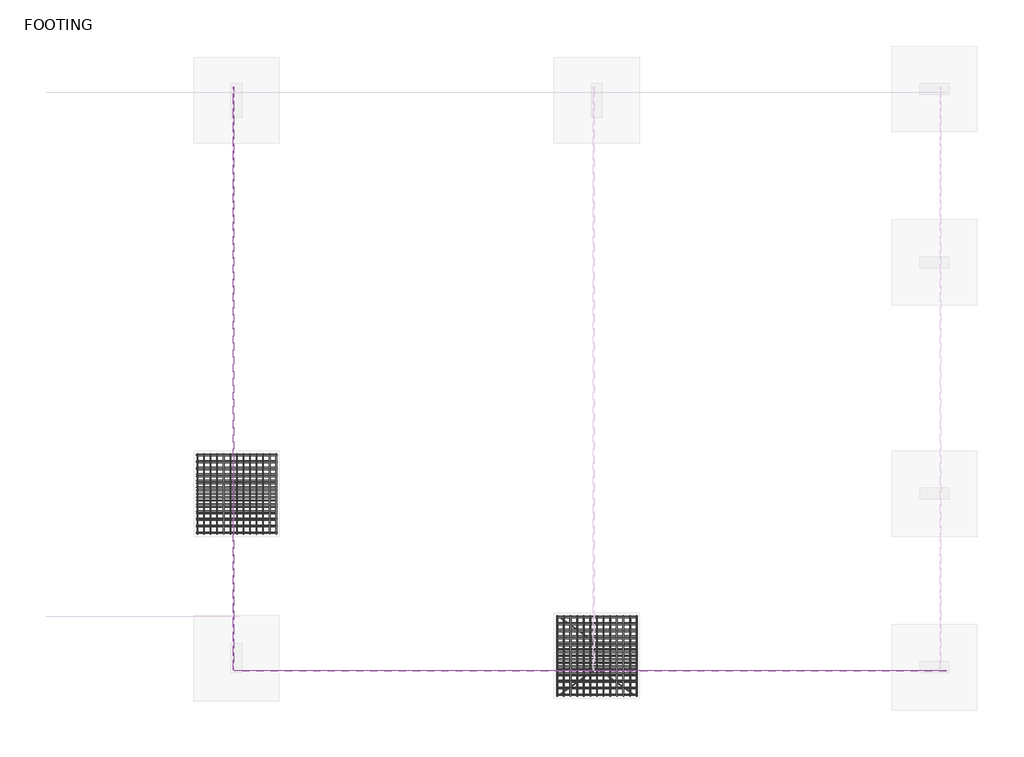
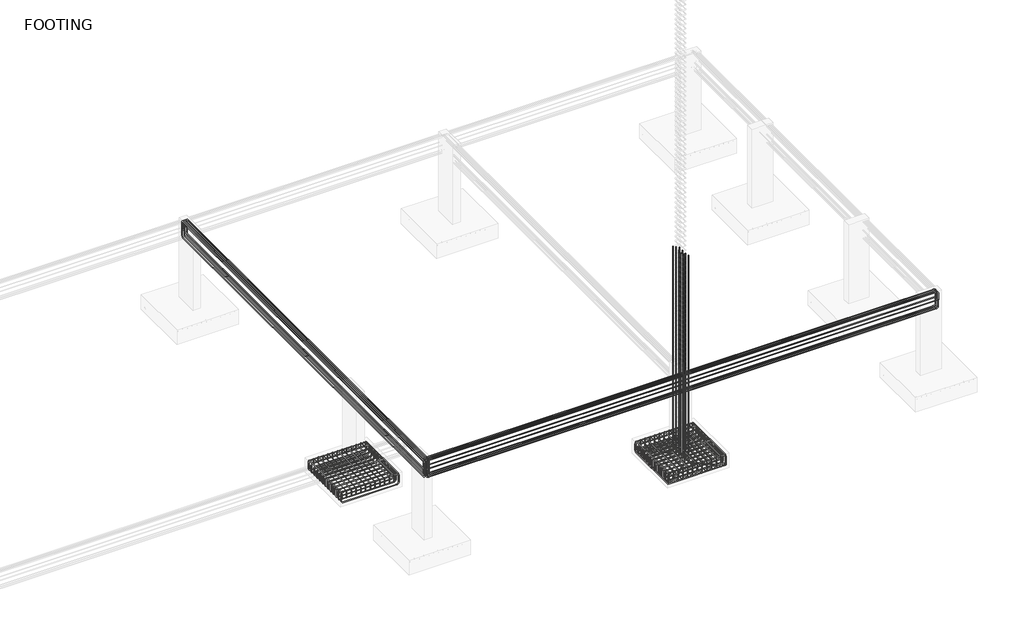
# One storey, part 6 of 12: 18 reinforcing bars.
"""IFC4 building model written with IfcOpenShell, lengths in millimetres."""

from ifc_helpers import new_model, si_unit, point, frame, origin, place, context, project, spatial, polyline, circle_curve, trimmed, segment, composite_curve, source, transform, mapped, element, save
from ifc_brep_helpers import swept_disk

model = new_model("IFC4")

# Units and contexts
model_context = context("Model", 3, world=origin())
ifc_project = project(units=[si_unit("LENGTHUNIT", "METRE", prefix="MILLI")], contexts=[model_context])

# Site, building, storey
site = spatial("IfcSite", under=ifc_project)
building = spatial("IfcBuilding", under=site)
storey = spatial("IfcBuildingStorey", under=building, Name="FOOTING", Elevation=-5638.8)

# Reinforcing bars
placement = place(None, origin())
reinforcing_bar_shape = source(origin(), model_context, "Body", "SolidModel", [
    swept_disk(composite_curve([segment(polyline([(12927.3998335, -14959.6541655, -5788.8), (12927.3998335, -14959.6541655, -5975.4)]), True, "CONTINUOUS"), segment(trimmed(circle_curve(frame((12927.3998335, -14904.2041655, -5975.4), z_axis=(1.0, 0.0, 0.0), x_axis=(0.0, -55.45000000000073, 0.0)), 55.45), [point((12927.3998335, -14959.6541655, -5975.4))], [point((12927.3998335, -14904.2041655, -6030.85))], True, "CARTESIAN"), True, "CONTINUOUS"), segment(polyline([(12927.3998335, -14904.2041655, -6030.85), (12927.3998335, -13331.0041655, -6030.85)]), True, "CONTINUOUS"), segment(trimmed(circle_curve(frame((12927.3998335, -13331.0041655, -5975.4), z_axis=(1.0, 0.0, 0.0), x_axis=(0.0, 0.0, -55.45000000000073)), 55.45), [point((12927.3998335, -13331.0041655, -6030.85))], [point((12927.3998335, -13275.5541655, -5975.4))], True, "CARTESIAN"), True, "CONTINUOUS"), segment(polyline([(12927.3998335, -13275.5541655, -5975.4), (12927.3998335, -13275.5541655, -5788.8)]), True, "CONTINUOUS")], self_intersect=False), 7.95),
])
element("IfcReinforcingBar", 1, at=placement, inside=storey, context=model_context, shape_type="MappedRepresentation", body=[
    mapped(reinforcing_bar_shape, transform((0.0, 0.0, 0.0), x_axis=(1.0, 0.0, 0.0), y_axis=(0.0, 1.0, 0.0), z_axis=(0.0, 0.0, 1.0))),
    mapped(reinforcing_bar_shape, transform((-140.3416667, 0.0, 0.0), x_axis=(1.0, 0.0, 0.0), y_axis=(0.0, 1.0, 0.0), z_axis=(0.0, 0.0, 1.0))),
    mapped(reinforcing_bar_shape, transform((-280.6833333, 0.0, 0.0), x_axis=(1.0, 0.0, 0.0), y_axis=(0.0, 1.0, 0.0), z_axis=(0.0, 0.0, 1.0))),
    mapped(reinforcing_bar_shape, transform((-421.025, 0.0, 0.0), x_axis=(1.0, 0.0, 0.0), y_axis=(0.0, 1.0, 0.0), z_axis=(0.0, 0.0, 1.0))),
    mapped(reinforcing_bar_shape, transform((-561.3666667, 0.0, 0.0), x_axis=(1.0, 0.0, 0.0), y_axis=(0.0, 1.0, 0.0), z_axis=(0.0, 0.0, 1.0))),
    mapped(reinforcing_bar_shape, transform((-701.7083333, 0.0, 0.0), x_axis=(1.0, 0.0, 0.0), y_axis=(0.0, 1.0, 0.0), z_axis=(0.0, 0.0, 1.0))),
    mapped(reinforcing_bar_shape, transform((-842.05, 0.0, 0.0), x_axis=(1.0, 0.0, 0.0), y_axis=(0.0, 1.0, 0.0), z_axis=(0.0, 0.0, 1.0))),
    mapped(reinforcing_bar_shape, transform((-982.3916667, 0.0, 0.0), x_axis=(1.0, 0.0, 0.0), y_axis=(0.0, 1.0, 0.0), z_axis=(0.0, 0.0, 1.0))),
    mapped(reinforcing_bar_shape, transform((-1122.7333333, 0.0, 0.0), x_axis=(1.0, 0.0, 0.0), y_axis=(0.0, 1.0, 0.0), z_axis=(0.0, 0.0, 1.0))),
    mapped(reinforcing_bar_shape, transform((-1263.075, 0.0, 0.0), x_axis=(1.0, 0.0, 0.0), y_axis=(0.0, 1.0, 0.0), z_axis=(0.0, 0.0, 1.0))),
    mapped(reinforcing_bar_shape, transform((-1403.4166667, 0.0, 0.0), x_axis=(1.0, 0.0, 0.0), y_axis=(0.0, 1.0, 0.0), z_axis=(0.0, 0.0, 1.0))),
    mapped(reinforcing_bar_shape, transform((-1543.7583333, 0.0, 0.0), x_axis=(1.0, 0.0, 0.0), y_axis=(0.0, 1.0, 0.0), z_axis=(0.0, 0.0, 1.0))),
    mapped(reinforcing_bar_shape, transform((-1684.1, 0.0, 0.0), x_axis=(1.0, 0.0, 0.0), y_axis=(0.0, 1.0, 0.0), z_axis=(0.0, 0.0, 1.0))),
])
reinforcing_bar_2_shape = source(origin(), model_context, "Body", "SolidModel", [
    swept_disk(composite_curve([segment(polyline([(12918.2597994, -13273.9541655, -5888.8), (12918.2597994, -13273.9541655, -5741.5)]), True, "CONTINUOUS"), segment(trimmed(circle_curve(frame((12918.2597994, -13320.3041655, -5741.5), z_axis=(1.0, 0.0, 0.0), x_axis=(0.0, 46.350000000000364, 0.0)), 46.35), [point((12918.2597994, -13273.9541655, -5741.5))], [point((12918.2597994, -13320.3041655, -5695.15))], True, "CARTESIAN"), True, "CONTINUOUS"), segment(polyline([(12918.2597994, -13320.3041655, -5695.15), (12918.2597994, -14914.9041655, -5695.15)]), True, "CONTINUOUS"), segment(trimmed(circle_curve(frame((12918.2597994, -14914.9041655, -5741.5), z_axis=(1.0, 0.0, 0.0), x_axis=(0.0, 0.0, 46.350000000000364)), 46.35), [point((12918.2597994, -14914.9041655, -5695.15))], [point((12918.2597994, -14961.2541655, -5741.5))], True, "CARTESIAN"), True, "CONTINUOUS"), segment(polyline([(12918.2597994, -14961.2541655, -5741.5), (12918.2597994, -14961.2541655, -5888.8)]), True, "CONTINUOUS")], self_intersect=False), 6.35),
])
element("IfcReinforcingBar", 2, at=placement, inside=storey, context=model_context, shape_type="MappedRepresentation", body=[
    mapped(reinforcing_bar_2_shape, transform((0.0, 0.0, 0.0), x_axis=(1.0, 0.0, 0.0), y_axis=(0.0, 1.0, 0.0), z_axis=(0.0, 0.0, 1.0))),
    mapped(reinforcing_bar_2_shape, transform((-138.4829293, 0.0, 0.0), x_axis=(1.0, 0.0, 0.0), y_axis=(0.0, 1.0, 0.0), z_axis=(0.0, 0.0, 1.0))),
    mapped(reinforcing_bar_2_shape, transform((-276.9658586, 0.0, 0.0), x_axis=(1.0, 0.0, 0.0), y_axis=(0.0, 1.0, 0.0), z_axis=(0.0, 0.0, 1.0))),
    mapped(reinforcing_bar_2_shape, transform((-415.4487879, 0.0, 0.0), x_axis=(1.0, 0.0, 0.0), y_axis=(0.0, 1.0, 0.0), z_axis=(0.0, 0.0, 1.0))),
    mapped(reinforcing_bar_2_shape, transform((-553.9317172, 0.0, 0.0), x_axis=(1.0, 0.0, 0.0), y_axis=(0.0, 1.0, 0.0), z_axis=(0.0, 0.0, 1.0))),
    mapped(reinforcing_bar_2_shape, transform((-692.4146465, 0.0, 0.0), x_axis=(1.0, 0.0, 0.0), y_axis=(0.0, 1.0, 0.0), z_axis=(0.0, 0.0, 1.0))),
    mapped(reinforcing_bar_2_shape, transform((-830.8975758, 0.0, 0.0), x_axis=(1.0, 0.0, 0.0), y_axis=(0.0, 1.0, 0.0), z_axis=(0.0, 0.0, 1.0))),
    mapped(reinforcing_bar_2_shape, transform((-969.3805051, 0.0, 0.0), x_axis=(1.0, 0.0, 0.0), y_axis=(0.0, 1.0, 0.0), z_axis=(0.0, 0.0, 1.0))),
    mapped(reinforcing_bar_2_shape, transform((-1107.8634344, 0.0, 0.0), x_axis=(1.0, 0.0, 0.0), y_axis=(0.0, 1.0, 0.0), z_axis=(0.0, 0.0, 1.0))),
    mapped(reinforcing_bar_2_shape, transform((-1246.3463637, 0.0, 0.0), x_axis=(1.0, 0.0, 0.0), y_axis=(0.0, 1.0, 0.0), z_axis=(0.0, 0.0, 1.0))),
    mapped(reinforcing_bar_2_shape, transform((-1384.8292929, 0.0, 0.0), x_axis=(1.0, 0.0, 0.0), y_axis=(0.0, 1.0, 0.0), z_axis=(0.0, 0.0, 1.0))),
    mapped(reinforcing_bar_2_shape, transform((-1523.3122222, 0.0, 0.0), x_axis=(1.0, 0.0, 0.0), y_axis=(0.0, 1.0, 0.0), z_axis=(0.0, 0.0, 1.0))),
    mapped(reinforcing_bar_2_shape, transform((-1661.7951515, 0.0, 0.0), x_axis=(1.0, 0.0, 0.0), y_axis=(0.0, 1.0, 0.0), z_axis=(0.0, 0.0, 1.0))),
])
reinforcing_bar_3_shape = source(origin(), model_context, "Body", "SolidModel", [
    swept_disk(composite_curve([segment(polyline([(11243.2998335, -14942.6041655, -5773.0), (11243.2998335, -14942.6041655, -5959.6)]), True, "CONTINUOUS"), segment(trimmed(circle_curve(frame((11298.7498335, -14942.6041655, -5959.6), z_axis=(0.0, -1.0, 0.0), x_axis=(-55.45000000000073, 0.0, 0.0)), 55.45), [point((11243.2998335, -14942.6041655, -5959.6))], [point((11298.7498335, -14942.6041655, -6015.05))], True, "CARTESIAN"), True, "CONTINUOUS"), segment(polyline([(11298.7498335, -14942.6041655, -6015.05), (12871.9498335, -14942.6041655, -6015.05)]), True, "CONTINUOUS"), segment(trimmed(circle_curve(frame((12871.9498335, -14942.6041655, -5959.6), z_axis=(0.0, -1.0, 0.0), x_axis=(0.0, 0.0, -55.44999999999982)), 55.45), [point((12871.9498335, -14942.6041655, -6015.05))], [point((12927.3998335, -14942.6041655, -5959.6))], True, "CARTESIAN"), True, "CONTINUOUS"), segment(polyline([(12927.3998335, -14942.6041655, -5959.6), (12927.3998335, -14942.6041655, -5773.0)]), True, "CONTINUOUS")], self_intersect=False), 7.95),
])
element("IfcReinforcingBar", 3, at=placement, inside=storey, context=model_context, shape_type="MappedRepresentation", body=[
    mapped(reinforcing_bar_3_shape, transform((0.0, 0.0, 0.0), x_axis=(1.0, 0.0, 0.0), y_axis=(0.0, 1.0, 0.0), z_axis=(0.0, 0.0, 1.0))),
    mapped(reinforcing_bar_3_shape, transform((0.0, 137.7402087, 0.0), x_axis=(1.0, 0.0, 0.0), y_axis=(0.0, 1.0, 0.0), z_axis=(0.0, 0.0, 1.0))),
    mapped(reinforcing_bar_3_shape, transform((0.0, 275.4804175, 0.0), x_axis=(1.0, 0.0, 0.0), y_axis=(0.0, 1.0, 0.0), z_axis=(0.0, 0.0, 1.0))),
    mapped(reinforcing_bar_3_shape, transform((0.0, 413.2206262, 0.0), x_axis=(1.0, 0.0, 0.0), y_axis=(0.0, 1.0, 0.0), z_axis=(0.0, 0.0, 1.0))),
    mapped(reinforcing_bar_3_shape, transform((0.0, 550.960835, 0.0), x_axis=(1.0, 0.0, 0.0), y_axis=(0.0, 1.0, 0.0), z_axis=(0.0, 0.0, 1.0))),
    mapped(reinforcing_bar_3_shape, transform((0.0, 688.7010437, 0.0), x_axis=(1.0, 0.0, 0.0), y_axis=(0.0, 1.0, 0.0), z_axis=(0.0, 0.0, 1.0))),
    mapped(reinforcing_bar_3_shape, transform((0.0, 826.4412525, 0.0), x_axis=(1.0, 0.0, 0.0), y_axis=(0.0, 1.0, 0.0), z_axis=(0.0, 0.0, 1.0))),
    mapped(reinforcing_bar_3_shape, transform((0.0, 964.1814612, 0.0), x_axis=(1.0, 0.0, 0.0), y_axis=(0.0, 1.0, 0.0), z_axis=(0.0, 0.0, 1.0))),
    mapped(reinforcing_bar_3_shape, transform((0.0, 1101.92167, 0.0), x_axis=(1.0, 0.0, 0.0), y_axis=(0.0, 1.0, 0.0), z_axis=(0.0, 0.0, 1.0))),
    mapped(reinforcing_bar_3_shape, transform((0.0, 1239.6618787, 0.0), x_axis=(1.0, 0.0, 0.0), y_axis=(0.0, 1.0, 0.0), z_axis=(0.0, 0.0, 1.0))),
    mapped(reinforcing_bar_3_shape, transform((0.0, 1377.4020875, 0.0), x_axis=(1.0, 0.0, 0.0), y_axis=(0.0, 1.0, 0.0), z_axis=(0.0, 0.0, 1.0))),
    mapped(reinforcing_bar_3_shape, transform((0.0, 1515.1422962, 0.0), x_axis=(1.0, 0.0, 0.0), y_axis=(0.0, 1.0, 0.0), z_axis=(0.0, 0.0, 1.0))),
    mapped(reinforcing_bar_3_shape, transform((0.0, 1652.882505, 0.0), x_axis=(1.0, 0.0, 0.0), y_axis=(0.0, 1.0, 0.0), z_axis=(0.0, 0.0, 1.0))),
])
reinforcing_bar_4_shape = source(origin(), model_context, "Body", "SolidModel", [
    swept_disk(composite_curve([segment(polyline([(11243.2998335, -13299.9399866, -5950.85), (11243.2998335, -13299.9399866, -5764.25)]), True, "CONTINUOUS"), segment(trimmed(circle_curve(frame((11298.7498335, -13299.9399866, -5764.25), z_axis=(0.0, 1.0, 0.0), x_axis=(-55.45000000000073, 0.0, 0.0)), 55.45), [point((11243.2998335, -13299.9399866, -5764.25))], [point((11298.7498335, -13299.9399866, -5708.8))], True, "CARTESIAN"), True, "CONTINUOUS"), segment(polyline([(11298.7498335, -13299.9399866, -5708.8), (12871.9498335, -13299.9399866, -5708.8)]), True, "CONTINUOUS"), segment(trimmed(circle_curve(frame((12871.9498335, -13299.9399866, -5764.25), z_axis=(0.0, 1.0, 0.0), x_axis=(0.0, 0.0, 55.44999999999982)), 55.45), [point((12871.9498335, -13299.9399866, -5708.8))], [point((12927.3998335, -13299.9399866, -5764.25))], True, "CARTESIAN"), True, "CONTINUOUS"), segment(polyline([(12927.3998335, -13299.9399866, -5764.25), (12927.3998335, -13299.9399866, -5950.85)]), True, "CONTINUOUS")], self_intersect=False), 7.95),
])
element("IfcReinforcingBar", 4, at=placement, inside=storey, context=model_context, shape_type="MappedRepresentation", body=[
    mapped(reinforcing_bar_4_shape, transform((0.0, 0.0, 0.0), x_axis=(1.0, 0.0, 0.0), y_axis=(0.0, 1.0, 0.0), z_axis=(0.0, 0.0, 1.0))),
    mapped(reinforcing_bar_4_shape, transform((0.0, -148.1882348, 0.0), x_axis=(1.0, 0.0, 0.0), y_axis=(0.0, 1.0, 0.0), z_axis=(0.0, 0.0, 1.0))),
    mapped(reinforcing_bar_4_shape, transform((0.0, -296.3764695, 0.0), x_axis=(1.0, 0.0, 0.0), y_axis=(0.0, 1.0, 0.0), z_axis=(0.0, 0.0, 1.0))),
    mapped(reinforcing_bar_4_shape, transform((0.0, -444.5647043, 0.0), x_axis=(1.0, 0.0, 0.0), y_axis=(0.0, 1.0, 0.0), z_axis=(0.0, 0.0, 1.0))),
    mapped(reinforcing_bar_4_shape, transform((0.0, -592.7529391, 0.0), x_axis=(1.0, 0.0, 0.0), y_axis=(0.0, 1.0, 0.0), z_axis=(0.0, 0.0, 1.0))),
    mapped(reinforcing_bar_4_shape, transform((0.0, -740.9411738, 0.0), x_axis=(1.0, 0.0, 0.0), y_axis=(0.0, 1.0, 0.0), z_axis=(0.0, 0.0, 1.0))),
    mapped(reinforcing_bar_4_shape, transform((0.0, -889.1294086, 0.0), x_axis=(1.0, 0.0, 0.0), y_axis=(0.0, 1.0, 0.0), z_axis=(0.0, 0.0, 1.0))),
    mapped(reinforcing_bar_4_shape, transform((0.0, -1037.3176434, 0.0), x_axis=(1.0, 0.0, 0.0), y_axis=(0.0, 1.0, 0.0), z_axis=(0.0, 0.0, 1.0))),
    mapped(reinforcing_bar_4_shape, transform((0.0, -1185.5058782, 0.0), x_axis=(1.0, 0.0, 0.0), y_axis=(0.0, 1.0, 0.0), z_axis=(0.0, 0.0, 1.0))),
    mapped(reinforcing_bar_4_shape, transform((0.0, -1333.6941129, 0.0), x_axis=(1.0, 0.0, 0.0), y_axis=(0.0, 1.0, 0.0), z_axis=(0.0, 0.0, 1.0))),
    mapped(reinforcing_bar_4_shape, transform((0.0, -1481.8823477, 0.0), x_axis=(1.0, 0.0, 0.0), y_axis=(0.0, 1.0, 0.0), z_axis=(0.0, 0.0, 1.0))),
    mapped(reinforcing_bar_4_shape, transform((0.0, -1630.0705825, 0.0), x_axis=(1.0, 0.0, 0.0), y_axis=(0.0, 1.0, 0.0), z_axis=(0.0, 0.0, 1.0))),
])
reinforcing_bar_5_shape = source(origin(), model_context, "Body", "SolidModel", [
    swept_disk(composite_curve([segment(polyline([(5323.6597994, -9857.6541655, -5888.8), (5323.6597994, -9857.6541655, -5741.5)]), True, "CONTINUOUS"), segment(trimmed(circle_curve(frame((5323.6597994, -9904.0041655, -5741.5), z_axis=(1.0, 0.0, 0.0), x_axis=(0.0, 46.350000000000364, 0.0)), 46.35), [point((5323.6597994, -9857.6541655, -5741.5))], [point((5323.6597994, -9904.0041655, -5695.15))], True, "CARTESIAN"), True, "CONTINUOUS"), segment(polyline([(5323.6597994, -9904.0041655, -5695.15), (5323.6597994, -11498.6041655, -5695.15)]), True, "CONTINUOUS"), segment(trimmed(circle_curve(frame((5323.6597994, -11498.6041655, -5741.5), z_axis=(1.0, 0.0, 0.0), x_axis=(0.0, 0.0, 46.350000000000364)), 46.35), [point((5323.6597994, -11498.6041655, -5695.15))], [point((5323.6597994, -11544.9541655, -5741.5))], True, "CARTESIAN"), True, "CONTINUOUS"), segment(polyline([(5323.6597994, -11544.9541655, -5741.5), (5323.6597994, -11544.9541655, -5888.8)]), True, "CONTINUOUS")], self_intersect=False), 6.35),
])
element("IfcReinforcingBar", 5, at=placement, inside=storey, context=model_context, shape_type="MappedRepresentation", body=[
    mapped(reinforcing_bar_5_shape, transform((0.0, 0.0, 0.0), x_axis=(1.0, 0.0, 0.0), y_axis=(0.0, 1.0, 0.0), z_axis=(0.0, 0.0, 1.0))),
    mapped(reinforcing_bar_5_shape, transform((-138.4829293, 0.0, 0.0), x_axis=(1.0, 0.0, 0.0), y_axis=(0.0, 1.0, 0.0), z_axis=(0.0, 0.0, 1.0))),
    mapped(reinforcing_bar_5_shape, transform((-276.9658586, 0.0, 0.0), x_axis=(1.0, 0.0, 0.0), y_axis=(0.0, 1.0, 0.0), z_axis=(0.0, 0.0, 1.0))),
    mapped(reinforcing_bar_5_shape, transform((-415.4487879, 0.0, 0.0), x_axis=(1.0, 0.0, 0.0), y_axis=(0.0, 1.0, 0.0), z_axis=(0.0, 0.0, 1.0))),
    mapped(reinforcing_bar_5_shape, transform((-553.9317172, 0.0, 0.0), x_axis=(1.0, 0.0, 0.0), y_axis=(0.0, 1.0, 0.0), z_axis=(0.0, 0.0, 1.0))),
    mapped(reinforcing_bar_5_shape, transform((-692.4146465, 0.0, 0.0), x_axis=(1.0, 0.0, 0.0), y_axis=(0.0, 1.0, 0.0), z_axis=(0.0, 0.0, 1.0))),
    mapped(reinforcing_bar_5_shape, transform((-830.8975758, 0.0, 0.0), x_axis=(1.0, 0.0, 0.0), y_axis=(0.0, 1.0, 0.0), z_axis=(0.0, 0.0, 1.0))),
    mapped(reinforcing_bar_5_shape, transform((-969.3805051, 0.0, 0.0), x_axis=(1.0, 0.0, 0.0), y_axis=(0.0, 1.0, 0.0), z_axis=(0.0, 0.0, 1.0))),
    mapped(reinforcing_bar_5_shape, transform((-1107.8634344, 0.0, 0.0), x_axis=(1.0, 0.0, 0.0), y_axis=(0.0, 1.0, 0.0), z_axis=(0.0, 0.0, 1.0))),
    mapped(reinforcing_bar_5_shape, transform((-1246.3463637, 0.0, 0.0), x_axis=(1.0, 0.0, 0.0), y_axis=(0.0, 1.0, 0.0), z_axis=(0.0, 0.0, 1.0))),
    mapped(reinforcing_bar_5_shape, transform((-1384.8292929, 0.0, 0.0), x_axis=(1.0, 0.0, 0.0), y_axis=(0.0, 1.0, 0.0), z_axis=(0.0, 0.0, 1.0))),
    mapped(reinforcing_bar_5_shape, transform((-1523.3122222, 0.0, 0.0), x_axis=(1.0, 0.0, 0.0), y_axis=(0.0, 1.0, 0.0), z_axis=(0.0, 0.0, 1.0))),
    mapped(reinforcing_bar_5_shape, transform((-1661.7951515, 0.0, 0.0), x_axis=(1.0, 0.0, 0.0), y_axis=(0.0, 1.0, 0.0), z_axis=(0.0, 0.0, 1.0))),
])
reinforcing_bar_6_shape = source(origin(), model_context, "Body", "SolidModel", [
    swept_disk(composite_curve([segment(polyline([(3648.6998335, -11526.3041655, -5773.0), (3648.6998335, -11526.3041655, -5959.6)]), True, "CONTINUOUS"), segment(trimmed(circle_curve(frame((3704.1498335, -11526.3041655, -5959.6), z_axis=(0.0, -1.0, 0.0), x_axis=(-55.45000000000027, 0.0, 0.0)), 55.45), [point((3648.6998335, -11526.3041655, -5959.6))], [point((3704.1498335, -11526.3041655, -6015.05))], True, "CARTESIAN"), True, "CONTINUOUS"), segment(polyline([(3704.1498335, -11526.3041655, -6015.05), (5277.3498335, -11526.3041655, -6015.05)]), True, "CONTINUOUS"), segment(trimmed(circle_curve(frame((5277.3498335, -11526.3041655, -5959.6), z_axis=(0.0, -1.0, 0.0), x_axis=(0.0, 0.0, -55.44999999999982)), 55.45), [point((5277.3498335, -11526.3041655, -6015.05))], [point((5332.7998335, -11526.3041655, -5959.6))], True, "CARTESIAN"), True, "CONTINUOUS"), segment(polyline([(5332.7998335, -11526.3041655, -5959.6), (5332.7998335, -11526.3041655, -5773.0)]), True, "CONTINUOUS")], self_intersect=False), 7.95),
])
element("IfcReinforcingBar", 6, at=placement, inside=storey, context=model_context, shape_type="MappedRepresentation", body=[
    mapped(reinforcing_bar_6_shape, transform((0.0, 0.0, 0.0), x_axis=(1.0, 0.0, 0.0), y_axis=(0.0, 1.0, 0.0), z_axis=(0.0, 0.0, 1.0))),
    mapped(reinforcing_bar_6_shape, transform((0.0, 137.7402087, 0.0), x_axis=(1.0, 0.0, 0.0), y_axis=(0.0, 1.0, 0.0), z_axis=(0.0, 0.0, 1.0))),
    mapped(reinforcing_bar_6_shape, transform((0.0, 275.4804175, 0.0), x_axis=(1.0, 0.0, 0.0), y_axis=(0.0, 1.0, 0.0), z_axis=(0.0, 0.0, 1.0))),
    mapped(reinforcing_bar_6_shape, transform((0.0, 413.2206262, 0.0), x_axis=(1.0, 0.0, 0.0), y_axis=(0.0, 1.0, 0.0), z_axis=(0.0, 0.0, 1.0))),
    mapped(reinforcing_bar_6_shape, transform((0.0, 550.960835, 0.0), x_axis=(1.0, 0.0, 0.0), y_axis=(0.0, 1.0, 0.0), z_axis=(0.0, 0.0, 1.0))),
    mapped(reinforcing_bar_6_shape, transform((0.0, 688.7010437, 0.0), x_axis=(1.0, 0.0, 0.0), y_axis=(0.0, 1.0, 0.0), z_axis=(0.0, 0.0, 1.0))),
    mapped(reinforcing_bar_6_shape, transform((0.0, 826.4412525, 0.0), x_axis=(1.0, 0.0, 0.0), y_axis=(0.0, 1.0, 0.0), z_axis=(0.0, 0.0, 1.0))),
    mapped(reinforcing_bar_6_shape, transform((0.0, 964.1814612, 0.0), x_axis=(1.0, 0.0, 0.0), y_axis=(0.0, 1.0, 0.0), z_axis=(0.0, 0.0, 1.0))),
    mapped(reinforcing_bar_6_shape, transform((0.0, 1101.92167, 0.0), x_axis=(1.0, 0.0, 0.0), y_axis=(0.0, 1.0, 0.0), z_axis=(0.0, 0.0, 1.0))),
    mapped(reinforcing_bar_6_shape, transform((0.0, 1239.6618787, 0.0), x_axis=(1.0, 0.0, 0.0), y_axis=(0.0, 1.0, 0.0), z_axis=(0.0, 0.0, 1.0))),
    mapped(reinforcing_bar_6_shape, transform((0.0, 1377.4020875, 0.0), x_axis=(1.0, 0.0, 0.0), y_axis=(0.0, 1.0, 0.0), z_axis=(0.0, 0.0, 1.0))),
    mapped(reinforcing_bar_6_shape, transform((0.0, 1515.1422962, 0.0), x_axis=(1.0, 0.0, 0.0), y_axis=(0.0, 1.0, 0.0), z_axis=(0.0, 0.0, 1.0))),
    mapped(reinforcing_bar_6_shape, transform((0.0, 1652.882505, 0.0), x_axis=(1.0, 0.0, 0.0), y_axis=(0.0, 1.0, 0.0), z_axis=(0.0, 0.0, 1.0))),
])
reinforcing_bar_7_shape = source(origin(), model_context, "Body", "SolidModel", [
    swept_disk(composite_curve([segment(polyline([(3648.6998335, -9883.6399866, -5950.85), (3648.6998335, -9883.6399866, -5764.25)]), True, "CONTINUOUS"), segment(trimmed(circle_curve(frame((3704.1498335, -9883.6399866, -5764.25), z_axis=(0.0, 1.0, 0.0), x_axis=(-55.45000000000027, 0.0, 0.0)), 55.45), [point((3648.6998335, -9883.6399866, -5764.25))], [point((3704.1498335, -9883.6399866, -5708.8))], True, "CARTESIAN"), True, "CONTINUOUS"), segment(polyline([(3704.1498335, -9883.6399866, -5708.8), (5277.3498335, -9883.6399866, -5708.8)]), True, "CONTINUOUS"), segment(trimmed(circle_curve(frame((5277.3498335, -9883.6399866, -5764.25), z_axis=(0.0, 1.0, 0.0), x_axis=(0.0, 0.0, 55.44999999999982)), 55.45), [point((5277.3498335, -9883.6399866, -5708.8))], [point((5332.7998335, -9883.6399866, -5764.25))], True, "CARTESIAN"), True, "CONTINUOUS"), segment(polyline([(5332.7998335, -9883.6399866, -5764.25), (5332.7998335, -9883.6399866, -5950.85)]), True, "CONTINUOUS")], self_intersect=False), 7.95),
])
element("IfcReinforcingBar", 7, at=placement, inside=storey, context=model_context, shape_type="MappedRepresentation", body=[
    mapped(reinforcing_bar_7_shape, transform((0.0, 0.0, 0.0), x_axis=(1.0, 0.0, 0.0), y_axis=(0.0, 1.0, 0.0), z_axis=(0.0, 0.0, 1.0))),
    mapped(reinforcing_bar_7_shape, transform((0.0, -148.1882348, 0.0), x_axis=(1.0, 0.0, 0.0), y_axis=(0.0, 1.0, 0.0), z_axis=(0.0, 0.0, 1.0))),
    mapped(reinforcing_bar_7_shape, transform((0.0, -296.3764695, 0.0), x_axis=(1.0, 0.0, 0.0), y_axis=(0.0, 1.0, 0.0), z_axis=(0.0, 0.0, 1.0))),
    mapped(reinforcing_bar_7_shape, transform((0.0, -444.5647043, 0.0), x_axis=(1.0, 0.0, 0.0), y_axis=(0.0, 1.0, 0.0), z_axis=(0.0, 0.0, 1.0))),
    mapped(reinforcing_bar_7_shape, transform((0.0, -592.7529391, 0.0), x_axis=(1.0, 0.0, 0.0), y_axis=(0.0, 1.0, 0.0), z_axis=(0.0, 0.0, 1.0))),
    mapped(reinforcing_bar_7_shape, transform((0.0, -740.9411738, 0.0), x_axis=(1.0, 0.0, 0.0), y_axis=(0.0, 1.0, 0.0), z_axis=(0.0, 0.0, 1.0))),
    mapped(reinforcing_bar_7_shape, transform((0.0, -889.1294086, 0.0), x_axis=(1.0, 0.0, 0.0), y_axis=(0.0, 1.0, 0.0), z_axis=(0.0, 0.0, 1.0))),
    mapped(reinforcing_bar_7_shape, transform((0.0, -1037.3176434, 0.0), x_axis=(1.0, 0.0, 0.0), y_axis=(0.0, 1.0, 0.0), z_axis=(0.0, 0.0, 1.0))),
    mapped(reinforcing_bar_7_shape, transform((0.0, -1185.5058782, 0.0), x_axis=(1.0, 0.0, 0.0), y_axis=(0.0, 1.0, 0.0), z_axis=(0.0, 0.0, 1.0))),
    mapped(reinforcing_bar_7_shape, transform((0.0, -1333.6941129, 0.0), x_axis=(1.0, 0.0, 0.0), y_axis=(0.0, 1.0, 0.0), z_axis=(0.0, 0.0, 1.0))),
    mapped(reinforcing_bar_7_shape, transform((0.0, -1481.8823477, 0.0), x_axis=(1.0, 0.0, 0.0), y_axis=(0.0, 1.0, 0.0), z_axis=(0.0, 0.0, 1.0))),
    mapped(reinforcing_bar_7_shape, transform((0.0, -1630.0705825, 0.0), x_axis=(1.0, 0.0, 0.0), y_axis=(0.0, 1.0, 0.0), z_axis=(0.0, 0.0, 1.0))),
])
element("IfcReinforcingBar", 8, at=placement, inside=storey, context=model_context, shape_type="SolidModel", body=[
    swept_disk(composite_curve([segment(polyline([(12139.4849117, -14414.7482567, 415.8066325), (12139.4849117, -14414.7482567, -5942.169349)]), True, "CONTINUOUS"), segment(trimmed(circle_curve(frame((12184.4838884, -14447.1487906, -5942.169349), z_axis=(-0.5843198177171824, -0.8115234750904984, 0.0), x_axis=(-44.99897670000064, 32.40053389999957, 0.0)), 55.45), [point((12139.4849117, -14414.7482567, -5942.169349))], [point((12184.4838884, -14447.1487906, -5997.619349))], True, "CARTESIAN"), True, "CONTINUOUS"), segment(polyline([(12184.4838884, -14447.1487906, -5997.619349), (12841.2214201, -14920.0183583, -5997.619349)]), True, "CONTINUOUS")], self_intersect=False), 7.95),
])
reinforcing_bar_8_shape = source(origin(), model_context, "Body", "SolidModel", [
    swept_disk(composite_curve([segment(polyline([(12140.0984639, -14266.9702313, 392.620059), (12140.0984639, -14266.9702313, -5942.169349)]), True, "CONTINUOUS"), segment(trimmed(circle_curve(frame((12195.5484639, -14266.9702313, -5942.169349), z_axis=(0.0, -1.0, 0.0), x_axis=(-55.45000000000073, 0.0, 0.0)), 55.45), [point((12140.0984639, -14266.9702313, -5942.169349))], [point((12195.5484639, -14266.9702313, -5997.619349))], True, "CARTESIAN"), True, "CONTINUOUS"), segment(polyline([(12195.5484639, -14266.9702313, -5997.619349), (12935.7281193, -14266.9702313, -5997.619349)]), True, "CONTINUOUS")], self_intersect=False), 7.95),
])
element("IfcReinforcingBar", 9, at=placement, inside=storey, context=model_context, shape_type="MappedRepresentation", body=[
    mapped(reinforcing_bar_8_shape, transform((0.0, 0.0, 0.0), x_axis=(1.0, 0.0, 0.0), y_axis=(0.0, 1.0, 0.0), z_axis=(0.0, 0.0, 1.0))),
    mapped(reinforcing_bar_8_shape, transform((0.0, 147.7377485, 0.0), x_axis=(1.0, 0.0, 0.0), y_axis=(0.0, 1.0, 0.0), z_axis=(0.0, 0.0, 1.0))),
    mapped(reinforcing_bar_8_shape, transform((0.0, 295.475497, 0.0), x_axis=(1.0, 0.0, 0.0), y_axis=(0.0, 1.0, 0.0), z_axis=(0.0, 0.0, 1.0))),
])
element("IfcReinforcingBar", 10, at=placement, inside=storey, context=model_context, shape_type="SolidModel", body=[
    swept_disk(composite_curve([segment(polyline([(12027.8173146, -14411.952396, 505.5084766), (12027.8173146, -14411.952396, -5942.169349)]), True, "CONTINUOUS"), segment(trimmed(circle_curve(frame((11982.8183379, -14444.3529299, -5942.169349), z_axis=(-0.5843198177172044, 0.8115234750904825, 0.0), x_axis=(44.99897670000064, 32.40053389999957, 0.0)), 55.45), [point((12027.8173146, -14411.952396, -5942.169349))], [point((11982.8183379, -14444.3529299, -5997.619349))], True, "CARTESIAN"), True, "CONTINUOUS"), segment(polyline([(11982.8183379, -14444.3529299, -5997.619349), (11322.1978185, -14920.0183583, -5997.619349)]), True, "CONTINUOUS")], self_intersect=False), 7.95),
])
element("IfcReinforcingBar", 11, at=placement, inside=storey, context=model_context, shape_type="SolidModel", body=[
    swept_disk(composite_curve([segment(polyline([(12031.011177, -13823.5930989, 367.9679278), (12031.011177, -13823.5930989, -5942.169349)]), True, "CONTINUOUS"), segment(trimmed(circle_curve(frame((11986.0122003, -13791.192565, -5942.169349), z_axis=(0.5843198177171605, 0.8115234750905143, 0.0), x_axis=(44.99897670000064, -32.40053390000139, 0.0)), 55.45), [point((12031.011177, -13823.5930989, -5942.169349))], [point((11986.0122003, -13791.192565, -5997.619349))], True, "CARTESIAN"), True, "CONTINUOUS"), segment(polyline([(11986.0122003, -13791.192565, -5997.619349), (11338.074442, -13324.6590827, -5997.619349)]), True, "CONTINUOUS")], self_intersect=False), 7.95),
])
reinforcing_bar_9_shape = source(origin(), model_context, "Body", "SolidModel", [
    swept_disk(composite_curve([segment(polyline([(12030.9748335, -13971.4947343, 444.000582), (12030.9748335, -13971.4947343, -5942.169349)]), True, "CONTINUOUS"), segment(trimmed(circle_curve(frame((11975.5248335, -13971.4947343, -5942.169349), z_axis=(0.0, 1.0, 0.0), x_axis=(55.45000000000073, 0.0, 0.0)), 55.45), [point((12030.9748335, -13971.4947343, -5942.169349))], [point((11975.5248335, -13971.4947343, -5997.619349))], True, "CARTESIAN"), True, "CONTINUOUS"), segment(polyline([(11975.5248335, -13971.4947343, -5997.619349), (11234.9715476, -13971.4947343, -5997.619349)]), True, "CONTINUOUS")], self_intersect=False), 7.95),
])
element("IfcReinforcingBar", 12, at=placement, inside=storey, context=model_context, shape_type="MappedRepresentation", body=[
    mapped(reinforcing_bar_9_shape, transform((0.0, 0.0, 0.0), x_axis=(1.0, 0.0, 0.0), y_axis=(0.0, 1.0, 0.0), z_axis=(0.0, 0.0, 1.0))),
    mapped(reinforcing_bar_9_shape, transform((0.0, -147.7377485, 0.0), x_axis=(1.0, 0.0, 0.0), y_axis=(0.0, 1.0, 0.0), z_axis=(0.0, 0.0, 1.0))),
    mapped(reinforcing_bar_9_shape, transform((0.0, -295.475497, 0.0), x_axis=(1.0, 0.0, 0.0), y_axis=(0.0, 1.0, 0.0), z_axis=(0.0, 0.0, 1.0))),
])
reinforcing_bar_10_shape = source(origin(), model_context, "Body", "SolidModel", [
    swept_disk(composite_curve([segment(polyline([(4456.0608222, -14430.7541655, -3500.1457532), (19451.7259175, -14430.7541655, -3500.1457532)]), True, "CONTINUOUS")], self_intersect=False), 7.95),
])
element("IfcReinforcingBar", 13, at=placement, inside=storey, context=model_context, shape_type="MappedRepresentation", body=[
    mapped(reinforcing_bar_10_shape, transform((0.0, 0.0, 0.0), x_axis=(1.0, 0.0, 0.0), y_axis=(0.0, 1.0, 0.0), z_axis=(0.0, 0.0, 1.0))),
    mapped(reinforcing_bar_10_shape, transform((0.0, 143.7, 0.0), x_axis=(1.0, 0.0, 0.0), y_axis=(0.0, 1.0, 0.0), z_axis=(0.0, 0.0, 1.0))),
])
reinforcing_bar_11_shape = source(origin(), model_context, "Body", "SolidModel", [
    swept_disk(composite_curve([segment(polyline([(4460.3985608, -14427.2248022, -3488.4293633), (4460.3985608, -14427.2248022, -3301.8293633)]), True, "CONTINUOUS"), segment(trimmed(circle_curve(frame((4515.8485608, -14427.2248022, -3301.8293633), z_axis=(0.0, 1.0, 0.0), x_axis=(-55.44999999999982, 0.0, 0.0)), 55.45), [point((4460.3985608, -14427.2248022, -3301.8293633))], [point((4515.8485608, -14427.2248022, -3246.3793633))], True, "CARTESIAN"), True, "CONTINUOUS"), segment(polyline([(4515.8485608, -14427.2248022, -3246.3793633), (19388.3512095, -14427.2248022, -3246.3793633)]), True, "CONTINUOUS"), segment(trimmed(circle_curve(frame((19388.3512095, -14427.2248022, -3301.8293633), z_axis=(0.0, 1.0, 0.0), x_axis=(0.0, 0.0, 55.44999999999982)), 55.45), [point((19388.3512095, -14427.2248022, -3246.3793633))], [point((19443.8012095, -14427.2248022, -3301.8293633))], True, "CARTESIAN"), True, "CONTINUOUS"), segment(polyline([(19443.8012095, -14427.2248022, -3301.8293633), (19443.8012095, -14427.2248022, -3488.4293633)]), True, "CONTINUOUS")], self_intersect=False), 7.95),
])
element("IfcReinforcingBar", 14, at=placement, inside=storey, context=model_context, shape_type="MappedRepresentation", body=[
    mapped(reinforcing_bar_11_shape, transform((0.0, 0.0, 0.0), x_axis=(1.0, 0.0, 0.0), y_axis=(0.0, 1.0, 0.0), z_axis=(0.0, 0.0, 1.0))),
    mapped(reinforcing_bar_11_shape, transform((0.0, 45.5470911, 0.0), x_axis=(1.0, 0.0, 0.0), y_axis=(0.0, 1.0, 0.0), z_axis=(0.0, 0.0, 1.0))),
    mapped(reinforcing_bar_11_shape, transform((0.0, 91.0941823, 0.0), x_axis=(1.0, 0.0, 0.0), y_axis=(0.0, 1.0, 0.0), z_axis=(0.0, 0.0, 1.0))),
    mapped(reinforcing_bar_11_shape, transform((0.0, 136.6412734, 0.0), x_axis=(1.0, 0.0, 0.0), y_axis=(0.0, 1.0, 0.0), z_axis=(0.0, 0.0, 1.0))),
])
reinforcing_bar_12_shape = source(origin(), model_context, "Body", "SolidModel", [
    swept_disk(composite_curve([segment(polyline([(4460.420257, -14427.2248022, -3512.3706367), (4460.420257, -14427.2248022, -3698.9706367)]), True, "CONTINUOUS"), segment(trimmed(circle_curve(frame((4515.870257, -14427.2248022, -3698.9706367), z_axis=(0.0, -1.0, 0.0), x_axis=(-55.44999999999982, 0.0, 0.0)), 55.45), [point((4460.420257, -14427.2248022, -3698.9706367))], [point((4515.870257, -14427.2248022, -3754.4206367))], True, "CARTESIAN"), True, "CONTINUOUS"), segment(polyline([(4515.870257, -14427.2248022, -3754.4206367), (19384.0310743, -14427.2248022, -3754.4206367)]), True, "CONTINUOUS"), segment(trimmed(circle_curve(frame((19384.0310743, -14427.2248022, -3698.9706367), z_axis=(0.0, -1.0, 0.0), x_axis=(0.0, 0.0, -55.45000000000027)), 55.45), [point((19384.0310743, -14427.2248022, -3754.4206367))], [point((19439.4810743, -14427.2248022, -3698.9706367))], True, "CARTESIAN"), True, "CONTINUOUS"), segment(polyline([(19439.4810743, -14427.2248022, -3698.9706367), (19439.4810743, -14427.2248022, -3512.3706367)]), True, "CONTINUOUS")], self_intersect=False), 7.95),
])
element("IfcReinforcingBar", 15, at=placement, inside=storey, context=model_context, shape_type="MappedRepresentation", body=[
    mapped(reinforcing_bar_12_shape, transform((0.0, 0.0, 0.0), x_axis=(1.0, 0.0, 0.0), y_axis=(0.0, 1.0, 0.0), z_axis=(0.0, 0.0, 1.0))),
    mapped(reinforcing_bar_12_shape, transform((0.0, 68.3206367, 0.0), x_axis=(1.0, 0.0, 0.0), y_axis=(0.0, 1.0, 0.0), z_axis=(0.0, 0.0, 1.0))),
    mapped(reinforcing_bar_12_shape, transform((0.0, 136.6412734, 0.0), x_axis=(1.0, 0.0, 0.0), y_axis=(0.0, 1.0, 0.0), z_axis=(0.0, 0.0, 1.0))),
])
reinforcing_bar_13_shape = source(origin(), model_context, "Body", "SolidModel", [
    swept_disk(composite_curve([segment(polyline([(4562.5998335, -14409.8048205, -3500.1457532), (4562.5998335, -2115.7280815, -3500.1457532)]), True, "CONTINUOUS")], self_intersect=False), 7.95),
])
element("IfcReinforcingBar", 16, at=placement, inside=storey, context=model_context, shape_type="MappedRepresentation", body=[
    mapped(reinforcing_bar_13_shape, transform((0.0, 0.0, 0.0), x_axis=(1.0, 0.0, 0.0), y_axis=(0.0, 1.0, 0.0), z_axis=(0.0, 0.0, 1.0))),
    mapped(reinforcing_bar_13_shape, transform((-143.7, 0.0, 0.0), x_axis=(1.0, 0.0, 0.0), y_axis=(0.0, 1.0, 0.0), z_axis=(0.0, 0.0, 1.0))),
])
reinforcing_bar_14_shape = source(origin(), model_context, "Body", "SolidModel", [
    swept_disk(composite_curve([segment(polyline([(4559.0704702, -14400.658483, -3488.4293633), (4559.0704702, -14400.658483, -3301.8293633)]), True, "CONTINUOUS"), segment(trimmed(circle_curve(frame((4559.0704702, -14345.208483, -3301.8293633), z_axis=(-1.0, 0.0, 0.0), x_axis=(0.0, -55.44999999999891, 0.0)), 55.45), [point((4559.0704702, -14400.658483, -3301.8293633))], [point((4559.0704702, -14345.208483, -3246.3793633))], True, "CARTESIAN"), True, "CONTINUOUS"), segment(polyline([(4559.0704702, -14345.208483, -3246.3793633), (4559.0704702, -2179.1027895, -3246.3793633)]), True, "CONTINUOUS"), segment(trimmed(circle_curve(frame((4559.0704702, -2179.1027895, -3301.8293633), z_axis=(-1.0, 0.0, 0.0), x_axis=(0.0, 0.0, 55.44999999999982)), 55.45), [point((4559.0704702, -2179.1027895, -3246.3793633))], [point((4559.0704702, -2123.6527895, -3301.8293633))], True, "CARTESIAN"), True, "CONTINUOUS"), segment(polyline([(4559.0704702, -2123.6527895, -3301.8293633), (4559.0704702, -2123.6527895, -3488.4293633)]), True, "CONTINUOUS")], self_intersect=False), 7.95),
])
element("IfcReinforcingBar", 17, at=placement, inside=storey, context=model_context, shape_type="MappedRepresentation", body=[
    mapped(reinforcing_bar_14_shape, transform((0.0, 0.0, 0.0), x_axis=(1.0, 0.0, 0.0), y_axis=(0.0, 1.0, 0.0), z_axis=(0.0, 0.0, 1.0))),
    mapped(reinforcing_bar_14_shape, transform((-45.5470911, 0.0, 0.0), x_axis=(1.0, 0.0, 0.0), y_axis=(0.0, 1.0, 0.0), z_axis=(0.0, 0.0, 1.0))),
    mapped(reinforcing_bar_14_shape, transform((-91.0941823, 0.0, 0.0), x_axis=(1.0, 0.0, 0.0), y_axis=(0.0, 1.0, 0.0), z_axis=(0.0, 0.0, 1.0))),
    mapped(reinforcing_bar_14_shape, transform((-136.6412734, 0.0, 0.0), x_axis=(1.0, 0.0, 0.0), y_axis=(0.0, 1.0, 0.0), z_axis=(0.0, 0.0, 1.0))),
])
reinforcing_bar_15_shape = source(origin(), model_context, "Body", "SolidModel", [
    swept_disk(composite_curve([segment(polyline([(4559.0704702, -14409.5370155, -3512.3706367), (4559.0704702, -14409.5370155, -3698.9706367)]), True, "CONTINUOUS"), segment(trimmed(circle_curve(frame((4559.0704702, -14354.0870155, -3698.9706367), z_axis=(1.0, 0.0, 0.0), x_axis=(0.0, -55.45000000000073, 0.0)), 55.45), [point((4559.0704702, -14409.5370155, -3698.9706367))], [point((4559.0704702, -14354.0870155, -3754.4206367))], True, "CARTESIAN"), True, "CONTINUOUS"), segment(polyline([(4559.0704702, -14354.0870155, -3754.4206367), (4559.0704702, -2183.4229247, -3754.4206367)]), True, "CONTINUOUS"), segment(trimmed(circle_curve(frame((4559.0704702, -2183.4229247, -3698.9706367), z_axis=(1.0, 0.0, 0.0), x_axis=(0.0, 0.0, -55.45000000000027)), 55.45), [point((4559.0704702, -2183.4229247, -3754.4206367))], [point((4559.0704702, -2127.9729247, -3698.9706367))], True, "CARTESIAN"), True, "CONTINUOUS"), segment(polyline([(4559.0704702, -2127.9729247, -3698.9706367), (4559.0704702, -2127.9729247, -3512.3706367)]), True, "CONTINUOUS")], self_intersect=False), 7.95),
])
element("IfcReinforcingBar", 18, at=placement, inside=storey, context=model_context, shape_type="MappedRepresentation", body=[
    mapped(reinforcing_bar_15_shape, transform((0.0, 0.0, 0.0), x_axis=(1.0, 0.0, 0.0), y_axis=(0.0, 1.0, 0.0), z_axis=(0.0, 0.0, 1.0))),
    mapped(reinforcing_bar_15_shape, transform((-68.3206367, 0.0, 0.0), x_axis=(1.0, 0.0, 0.0), y_axis=(0.0, 1.0, 0.0), z_axis=(0.0, 0.0, 1.0))),
    mapped(reinforcing_bar_15_shape, transform((-136.6412734, 0.0, 0.0), x_axis=(1.0, 0.0, 0.0), y_axis=(0.0, 1.0, 0.0), z_axis=(0.0, 0.0, 1.0))),
])

save(model, "model.ifc")

# Revit data of these elements
# Elements 1, 2, 3, 4, 5, 6, 7, 8, 9, 10, 11, 12, 13, 14, 15, 16, 17, 18 (IfcReinforcingBar)
#   Phase Created = New Construction
